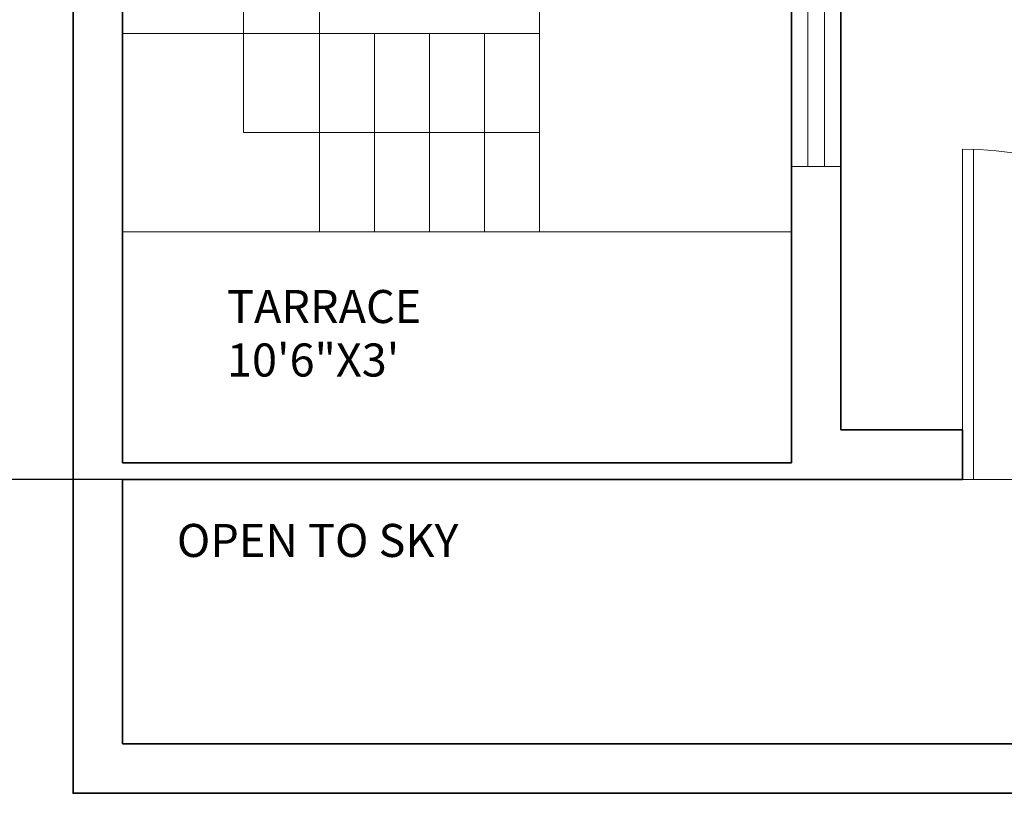
# Model space of a CAD drawing. Units: inches. Extents: x 125 to 976, y 231 to 853.
# Tile 12 of 16: x 557 to 736, y 272 to 413. Entities that reach past the tile are written whole.
import ezdxf

# ---------------------------------------------------------------- set-up
doc = ezdxf.new("R2010")
doc.units = ezdxf.units.IN
doc.header["$MEASUREMENT"] = 0
for name, color, linetype, lineweight in [('A-ANNO-DIMS', 2, 'Continuous', 18), ('A-AREA-IDEN', 7, 'Continuous', 18), ('A-DOOR', 3, 'Continuous', 18), ('A-FLOR', 8, 'Continuous', 18), ('A-FLOR-STRS', 7, 'Continuous', 18), ('A-GLAZ', 4, 'Continuous', 18), ('A-WALL', 7, 'Continuous', 35)]:
    doc.layers.add(name, color=color, linetype=linetype, lineweight=lineweight)
doc.styles.get("Standard").update_dxf_attribs({"font": 'italic8.shx'})
doc.dimstyles.get("Standard").update_dxf_attribs({"dimtxt": 8, "dimasz": 0.18, "dimexe": 0.18, "dimexo": 0.0625, "dimgap": 0.09, "dimtad": 0, "dimtih": 1, "dimtoh": 1, "dimdec": 4, "dimzin": 0, "dimdsep": 46, "dimlunit": 3, "dimtxsty": 'Standard', "dimcen": 0.09, "dimclrt": 4, "dimadec": 0, "dimazin": 0, "dimtfac": 1, "dimtdec": 4, "dimtofl": 0, "dimtmove": 0, "dimatfit": 3, "dimfxl": 1, "dimtolj": 1, "dimtzin": 0, "dimarcsym": 0})

# ---------------------------------------------------------------- blocks, each defined once
blk = doc.blocks.new('WINDOW-48IN')
for p, q in [((0, 0), (0, 48)), ((0, 48), (9, 48)), ((3, 0), (3, 48)), ((6, 0), (6, 48)), ((9, 48), (9, 0)), ((9, 0), (0, 0))]:
    blk.add_line(p, q)
blk = doc.blocks.new('DOOR-60IN')
for p, q in [((0, 0), (0, 60)), ((2, 0), (2, 59.97)), ((60, 0), (0, 0))]:
    blk.add_line(p, q)
blk.add_arc((0, 0), 60, 0, 90)
blk = doc.blocks.new('*D57')
at = {"layer": 'A-ANNO-DIMS', "color": 0, "lineweight": -2, "transparency": 16777216}
for p, q in [((567.13, 812.1), (538.31, 812.1)), ((538.49, 811.92), (538.49, 575.46)), ((538.49, 329.28), (538.49, 565.75)), ((576.13, 329.1), (538.31, 329.1))]:
    blk.add_line(p, q, dxfattribs=at)
at = {"layer": 'A-ANNO-DIMS', "color": 0, "transparency": 16777216}
for points in [[(538.46, 811.92), (538.52, 811.92), (538.49, 812.1)], [(538.46, 329.28), (538.52, 329.28), (538.49, 329.1)]]:
    blk.add_solid(points, dxfattribs=at)
at = {"layer": 'Defpoints', "color": 0, "transparency": 16777216}
for p in [(538.49, 812.1), (567.19, 812.1), (576.19, 329.1)]:
    blk.add_point(p, dxfattribs=at)
at = {"layer": 'A-ANNO-DIMS', "color": 4, "transparency": 16777216, "insert": (538.49, 570.6), "char_height": 8, "attachment_point": 5}
blk.add_mtext('\\A1;40\'-3"', dxfattribs=at)

msp = doc.modelspace()

# ---------------------------------------------------------------- linework, layer by layer
at = {"layer": 'A-FLOR'}
msp.add_line((697.69287, 374.10475), (576.19287, 374.10475), dxfattribs=at)
at = {"layer": 'A-FLOR-STRS'}
for p, q in [((598.15361, 392.10475), (598.15361, 476.58328)), ((611.96359, 374.10475), (611.96359, 462.17207)), ((651.96359, 462.17207), (651.96359, 410.10475)), ((611.96359, 410.10475), (576.19287, 410.10475)), ((651.96359, 410.10475), (611.96359, 410.10475)), ((621.96359, 374.10475), (621.96359, 410.10475)), ((631.96359, 374.10475), (631.96359, 410.10475)), ((641.96359, 374.10475), (641.96359, 410.10475)), ((651.96359, 374.10475), (651.96359, 410.10475)), ((651.96359, 392.10475), (598.15361, 392.10475))]:
    msp.add_line(p, q, dxfattribs=at)
at = {"layer": 'A-WALL'}
for p, q in [((576.19287, 332.10475), (576.19287, 494.10475)), ((697.69287, 494.10475), (697.69287, 332.10475)), ((706.69287, 494.10475), (706.69287, 338.10475)), ((728.78314, 338.10475), (706.69287, 338.10475)), ((728.78314, 338.10475), (728.78314, 329.10475)), ((697.69287, 332.10475), (576.19287, 332.10475)), ((576.19287, 281.10475), (576.19287, 329.10475)), ((728.78314, 329.10475), (576.19287, 329.10475)), ((846.19287, 281.10475), (576.19287, 281.10475))]:
    msp.add_line(p, q, dxfattribs=at)
msp.add_lwpolyline([(567.19287, 812.10475), (855.19287, 812.10475), (855.19287, 272.10475), (567.19287, 272.10475)], close=True, dxfattribs=at)

# ---------------------------------------------------------------- block references
at = {"layer": 'A-DOOR'}
msp.add_blockref('DOOR-60IN', (728.78314, 329.10475), dxfattribs=at)
at = {"layer": 'A-GLAZ'}
msp.add_blockref('WINDOW-48IN', (697.69, 385.91728), dxfattribs=at)

# ---------------------------------------------------------------- texts
at = {"layer": 'A-AREA-IDEN'}
for s, p in [('TARRACE', (595.16768, 357.51394)), ('10\'6"X3\'', (595.16768, 347.79965)), ('OPEN TO SKY', (586.05604, 315.02823))]:
    msp.add_text(s, height=6, dxfattribs=at).set_placement(p)

# ---------------------------------------------------------------- dimensions: what is measured, and where the dimension line sits
at = {"layer": 'A-ANNO-DIMS'}
dim = msp.add_linear_dim(base=(538.49287, 812.10475), p1=(576.19287, 329.10475), p2=(567.19287, 812.10475), angle=90, dimstyle='Standard', override={"dimdec": 1, "dimlfac": 1, "dimrnd": 0, "dimzin": 1, "dimdsep": 46, "dimlunit": 4, "dimfrac": 2}, dxfattribs=at)
dim.commit()
dim.dimension.update_dxf_attribs({"geometry": '*D57', "text_midpoint": (538.49287, 570.60475)})

doc.saveas('drawing.dxf')
